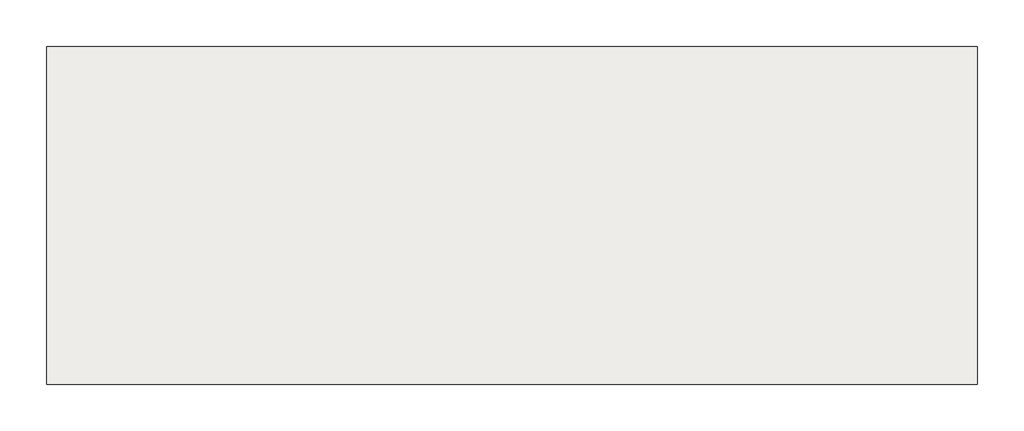
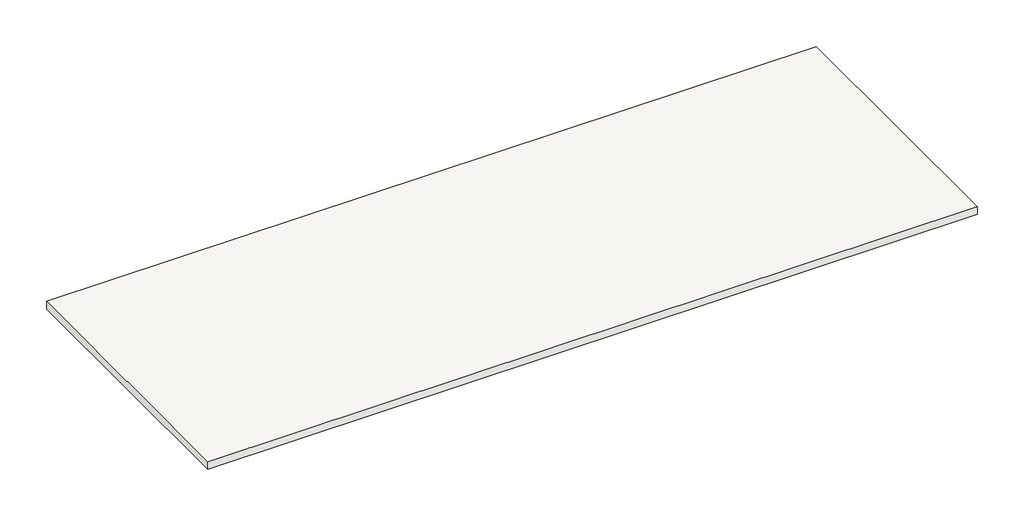
# One storey: 1 slab.
"""IFC4 building model written with IfcOpenShell, lengths in millimetres."""

from ifc_helpers import new_model, si_unit, frame, origin, place, context, project, spatial, polyline, outline, extrude, element, save

model = new_model("IFC4")

# Units and contexts
model_context = context("Model", 3, world=origin())
ifc_project = project(units=[si_unit("LENGTHUNIT", "METRE", prefix="MILLI")], contexts=[model_context])

# Site, building, storey
site = spatial("IfcSite", under=ifc_project)
building = spatial("IfcBuilding", under=site)
storey = spatial("IfcBuildingStorey", under=building, Elevation=-152.4)

# Slab
placement = place(None, origin())
element("IfcSlab", 1, at=placement, inside=storey, context=model_context, shape_type="SweptSolid", body=[
    extrude(outline(polyline([(18217.5782182, -6719.3758122), (18217.5782182, -9335.5758122), (11011.2916032, -9335.5758122), (11011.2916032, -6719.3758122), (18217.5782182, -6719.3758122)])), frame((0.0, 0.0, -381.0), z_axis=(0.0, 0.0, 1.0), x_axis=(1.0, 0.0, 0.0)), (0.0, 0.0, 1.0), 76.2),
])

save(model, "model.ifc")

# Revit data of these elements
# Type
#   Assembly Code = "B1010"
#   Function = 0
#   Layers, outside or top first: 0' - 1" "sand" (function 4); 0' - 2" "Wall Material (1)" (function 1)
# Element 1 (IfcSlab)
#   Height Offset From Level = -0' - 6"
#   Phase Created = A10 - Substructure
#   Materials on its faces: "Wall Material (1)", "sand"
# Materials
#   "sand": class "Generic", colour RGB 80 58 38, transparency 0, Cost = 0
#   "Wall Material (1)": colour RGB 127 127 127, transparency 0, Cost = 0
